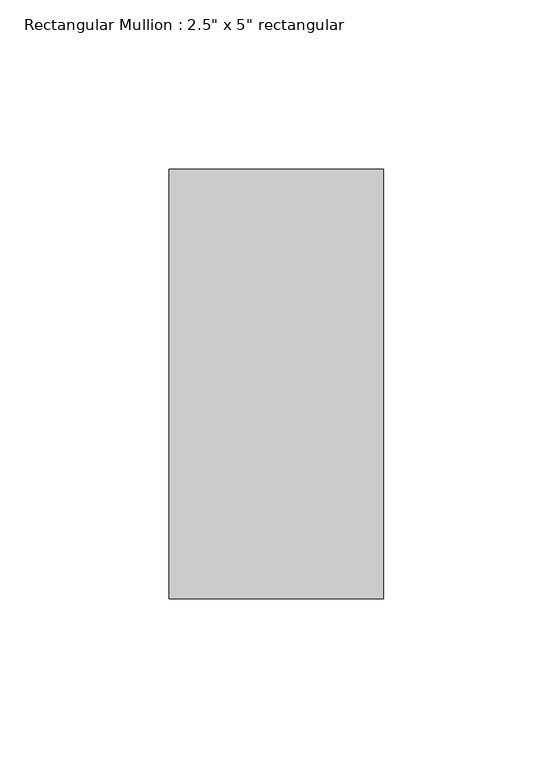
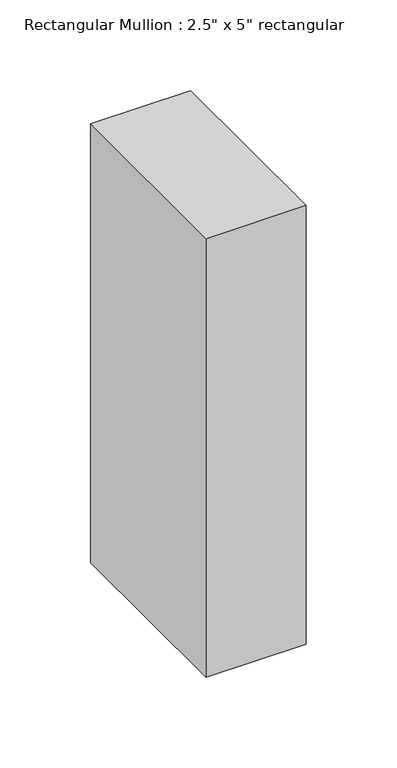
"""IFC4 building model written with IfcOpenShell, lengths in millimetres: member geometry."""

from ifc_helpers import new_model, si_unit, frame, origin, place, context, project, spatial, polyline, outline, extrude, source, transform, mapped, element, save


def member_5d039c20(model_context):
    return source(origin(), model_context, "Body", "SweptSolid", [
        extrude(outline(polyline([(31.75, 63.5), (31.75, -63.5), (-31.75, -63.5), (-31.75, 63.5), (31.75, 63.5)])), frame((0.0, 0.0, -294.64), z_axis=(0.0, 0.0, 1.0), x_axis=(1.0, 0.0, 0.0)), (0.0, 0.0, 1.0), 294.64),
    ])


if __name__ == "__main__":
    model = new_model("IFC4")
    model_context = context("Model", 3, world=origin())
    ifc_project = project(units=[si_unit("LENGTHUNIT", "METRE", prefix="MILLI")], contexts=[model_context])
    site = spatial("IfcSite", under=ifc_project)
    building = spatial("IfcBuilding", under=site)
    placement = place(None, origin())
    member_shape = member_5d039c20(model_context)
    element("IfcMember", 1, ObjectType="Rectangular Mullion : 2.5\" x 5\" rectangular", at=placement, inside=building, context=model_context, shape_type="MappedRepresentation", body=[
        mapped(member_shape, transform((0.0, 0.0, 0.0), x_axis=(1.0, 0.0, 0.0), y_axis=(0.0, 1.0, 0.0), z_axis=(0.0, 0.0, 1.0))),
    ])
    save(model, "model.ifc")

# Revit data of these elements
# Type "Rectangular Mullion : 2.5\" x 5\" rectangular"
#   built-in parameter 1007304 = 0.416667 (stored number, unit not read)
#   built-in parameter 1007301 = 0.104167 (stored number, unit not read)
#   built-in parameter 1007300 = 0.104167 (stored number, unit not read)
# Element 1 (IfcMember, "Rectangular Mullion : 2.5\" x 5\" rectangular")
#   Materials on its faces: "Aluminum"
# Materials
#   "Aluminum": class "Metal", colour RGB 247 247 247, transparency 0, Description = "Aluminum 6061", Cost = 0
